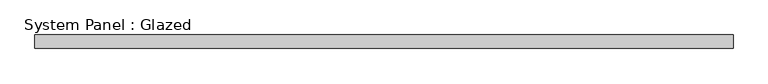
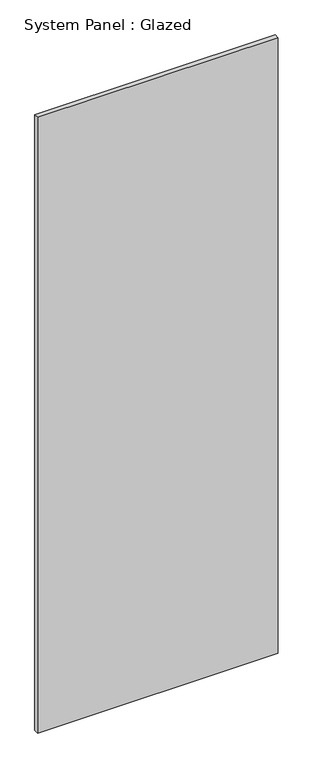
"""IFC4 building model written with IfcOpenShell, lengths in millimetres: plate geometry, System Panel : Glazed."""

from ifc_helpers import new_model, si_unit, origin, origin_with_axes, place, context, project, spatial, polyline, outline, extrude, source, transform, mapped, element, save


def system_panel_glazed_7496e499(model_context):
    return source(origin(), model_context, "Body", "SweptSolid", [
        extrude(outline(polyline([(652.6827143, 19.05), (-652.6827143, 19.05), (-652.6827143, 44.45), (652.6827143, 44.45), (652.6827143, 19.05)])), origin_with_axes(), (0.0, 0.0, 1.0), 3530.6),
    ])


if __name__ == "__main__":
    model = new_model("IFC4")
    model_context = context("Model", 3, world=origin())
    ifc_project = project(units=[si_unit("LENGTHUNIT", "METRE", prefix="MILLI")], contexts=[model_context])
    site = spatial("IfcSite", under=ifc_project)
    building = spatial("IfcBuilding", under=site)
    placement = place(None, origin())
    system_panel_glazed_shape = system_panel_glazed_7496e499(model_context)
    element("IfcPlate", 1, ObjectType="System Panel : Glazed", at=placement, inside=building, context=model_context, shape_type="MappedRepresentation", body=[
        mapped(system_panel_glazed_shape, transform((0.0, 0.0, 0.0), x_axis=(1.0, 0.0, 0.0), y_axis=(0.0, 1.0, 0.0), z_axis=(0.0, 0.0, 1.0))),
    ])
    save(model, "model.ifc")

# Revit data of these elements
# Type "System Panel : Glazed"
#   Construction Type Id = "GSP4R"
#   Analytic Construction = "1/8 in Pilkington single glazing"
#   Visual Light Transmittance = 0.9
#   Solar Heat Gain Coefficient = 0.86
#   Heat Transfer Coefficient (U) = 1.18115 BTU/(h·ft²·°F)
# Element 1 (IfcPlate, "System Panel : Glazed")
#   Materials on its faces: "Glass"
# Materials
#   "Glass": class "Glass", colour RGB 0 128 192, transparency 0.75, Description = "Soda Lime Glass", Cost = 0
